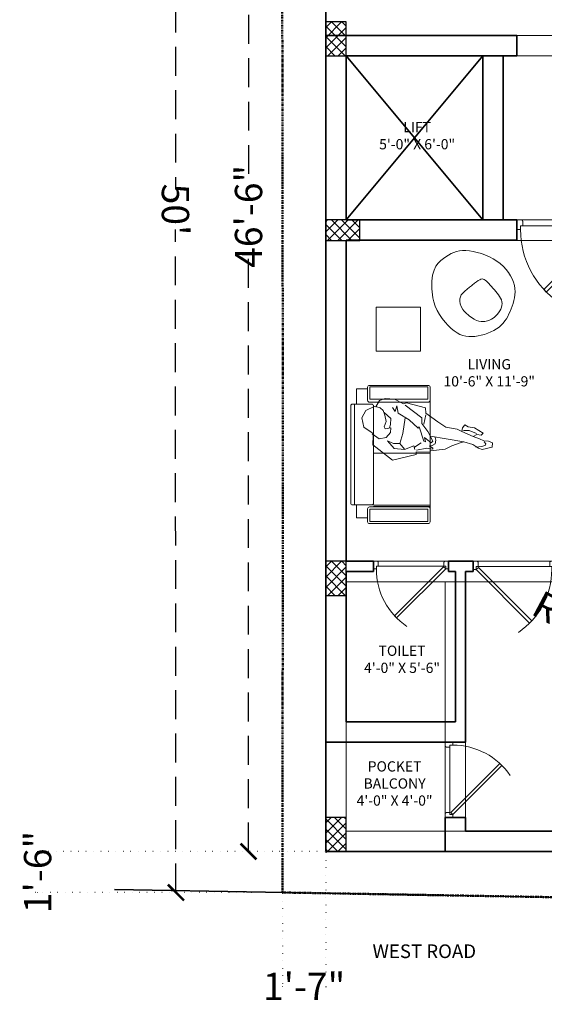
# Model space of a CAD drawing. Units: inches. Extents: x -16911 to -9621, y -48626 to -46270.
# Tile 17 of 20: x -11596 to -11365, y -47012 to -46579. Entities that reach past the tile are written whole.
import ezdxf

# ---------------------------------------------------------------- set-up
doc = ezdxf.new("R2010")
doc.units = ezdxf.units.IN
for name, pattern in [('DASHDOT', [1, 0.5, -0.25, 0, -0.25]), ('DASHED', [19.05, 12.7, -6.35]), ('DOT2', [3.175, 0, -3.175])]:
    doc.linetypes.add(name, pattern=pattern)
for name, color, linetype, lineweight in [('A-ANNO-DIMS', 2, 'Continuous', 13), ('A-ANNO-TEXT', 7, 'Continuous', 18), ('A-AREA-IDEN', 3, 'Continuous', 18), ('A-DOOR', 4, 'Continuous', 18), ('A-FURN', 8, 'Continuous', 13), ('A-WALL', 7, 'Continuous', 35), ('C-PROP', 6, 'DASHDOT', 50), ('column', 12, 'Continuous', 30), ('DOOR', 143, 'Continuous', 9), ('EXT BEAM', 132, 'Continuous', 13), ('furniture', 35, 'Continuous', 15), ('Man', 8, 'Continuous', 5), ('S-BEAM', 132, 'Continuous', 25), ('S-COLS', 1, 'Continuous', 30)]:
    doc.layers.add(name, color=color, linetype=linetype, lineweight=lineweight)
doc.styles.add('style9', font='swisscl.ttf', dxfattribs={"height": 12})
doc.dimstyles.new('Dim9', dxfattribs={"dimtxt": 10, "dimasz": 0.199219, "dimexe": 1, "dimexo": 0.5, "dimgap": 1, "dimtad": 0, "dimdec": 1, "dimzin": 0, "dimdsep": 46, "dimlunit": 4, "dimtxsty": 'style9', "dimblk": 'ARCHTICK', "dimcen": 0.09, "dimclrd": 256, "dimclrt": 256, "dimadec": 0, "dimazin": 0, "dimtfac": 1, "dimtdec": 1, "dimtix": 1, "dimtofl": 0, "dimtmove": 1, "dimatfit": 3, "dimfxl": 9, "dimtolj": 1, "dimtzin": 0, "dimlwd": -1, "dimarcsym": 0})

# ---------------------------------------------------------------- blocks, each defined once
blk = doc.blocks.new('Bipman02')
blk.add_lwpolyline([(0.5871, -0.067), (0.6175, -0.0496), (0.6523, -0.0539), (0.6697, -0.0376), (0.5958, 0.0069), (0.5437, 0.0156), (0.5164, 0.0297), (0.4959, 0.0069), (0.4915, -0.0235), (0.4524, -0.0061), (0.3568, 0.0113), (0.2917, 0.0548), (0.1917, 0.1287), (0.1874, 0.1722), (0.031, 0.2156), (0.0049, 0.2069), (-0.0689, 0.2461), (-0.1471, 0.2504), (-0.1949, 0.233), (-0.2253, 0.1808), (-0.2384, 0.1852), (-0.3079, 0.1504), (-0.3426, 0.0895), (-0.3253, 0.0113), (-0.2558, -0.0365), (-0.2471, -0.0583), (-0.2514, -0.1365), (-0.0863, -0.2626), (0.1092, -0.2148), (0.1092, -0.193), (0.2265, -0.1974), (0.2308, -0.1844), (0.3525, -0.1713), (0.409, -0.1452), (0.4872, -0.1148), (0.5089, -0.1104), (0.5828, -0.1322), (0.6088, -0.1496), (0.6295, -0.1636), (0.661, -0.1757), (0.7435, -0.1539), (0.7478, -0.1191), (0.7143, -0.1051), (0.674, -0.1017), (0.6392, -0.0844)], close=True)
for points in [[(-0.2558, -0.0452), (-0.1993, -0.0844), (-0.1385, -0.0757), (-0.1037, -0.0322), (-0.0994, 0.0069), (-0.1471, -0.0018), (-0.1558, 0.0156), (-0.1385, 0.0591), (-0.1515, 0.1113), (-0.1645, 0.1504), (-0.1906, 0.1722), (-0.2167, 0.1808)], [(-0.0863, 0.1765), (-0.0646, 0.1417), (-0.0516, 0.1895), (-0.0385, 0.1287), (0.0527, 0.0722), (0.1266, 0.0026), (0.1353, 0.0156), (0.1744, -0.1061), (0.1874, -0.1104), (0.1787, -0.0757), (0.2352, -0.1191), (0.2482, -0.1061), (0.2091, -0.0235), (0.157, 0.0417), (0.157, 0.0895), (0.018, 0.1939)], [(-0.1558, 0.133), (-0.0994, 0.0852), (-0.1037, 0.033), (-0.1124, 0.0069)], [(0.018, 0.0895), (0.0006, -0.0409), (-0.0255, -0.1235), (-0.0776, -0.1235), (-0.1298, -0.1017), (-0.0733, -0.167), (0.0136, -0.1757), (0.0918, -0.1452), (0.1005, -0.1757)], [(0.1917, 0.1156), (0.1744, 0.0374)], [(0.2699, -0.0757), (0.2743, -0.0974), (0.2699, -0.1278), (0.2439, -0.1409), (0.2222, -0.1452), (0.2482, -0.1626), (0.2482, -0.1713), (0.2004, -0.1626), (0.1135, -0.18)], [(0.2308, -0.0626), (0.3612, -0.0844), (0.5089, -0.1095)], [(0.4915, -0.0235), (0.5871, -0.067)], [(0.5045, -0.0148), (0.5523, -0.0148), (0.6132, -0.0409)], [(-0.0255, -0.1235), (0.0136, -0.1713)], [(0.0962, -0.1539), (0.1526, -0.1191)], [(0.6783, -0.1104), (0.6914, -0.1278), (0.687, -0.1409), (0.6566, -0.1496), (0.6088, -0.1539)]]:
    blk.add_lwpolyline(points)
blk = doc.blocks.new('erertety')
at = {"layer": 'furniture', "ltscale": 0.2}
for p, q in [((-17662.13, -45230.66), (-17662.13, -45176.69)), ((-17693.83, -45223.2), (-17693.83, -45184.43)), ((-17685.49, -45183.68), (-17693.08, -45183.68)), ((-17684.74, -45223.2), (-17684.74, -45184.43)), ((-17684.74, -45203.31), (-17662.13, -45203.31)), ((-17685.49, -45223.95), (-17693.08, -45223.95)), ((-17691.58, -45223.95), (-17691.58, -45229.1)), ((-17684.74, -45223.99), (-17662.13, -45223.99)), ((-17684.74, -45224.55), (-17662.13, -45224.55)), ((-17684.74, -45224.55), (-17662.13, -45224.55)), ((-17691.58, -45229.1), (-17687.09, -45229.1))]:
    blk.add_line(p, q, dxfattribs=at)
for points in [[(-17662.13, -45182.17), (-17662.13, -45176.97, 0.414214), (-17662.87, -45176.22), (-17686.34, -45176.22, 0.414214), (-17687.09, -45176.97), (-17687.09, -45182.17, 0.414214), (-17686.34, -45182.91), (-17662.87, -45182.91, 0.414214)], [(-17662.13, -45225.47), (-17662.13, -45230.66, -0.414214), (-17662.87, -45231.41), (-17686.34, -45231.41, -0.414214), (-17687.09, -45230.66), (-17687.09, -45225.47, -0.414214), (-17686.34, -45224.72), (-17662.87, -45224.72, -0.414214)]]:
    blk.add_lwpolyline(points, format="xyb", close=True, dxfattribs=at)
for points in [[(-17663.01, -45181.75), (-17663.01, -45176.82), (-17686.21, -45176.82), (-17686.21, -45181.75)], [(-17692.4, -45183.68), (-17692.4, -45223.95), (-17692.4, -45223.95), (-17692.4, -45183.68)], [(-17663.01, -45225.6), (-17663.01, -45230.53), (-17686.21, -45230.53), (-17686.21, -45225.6)]]:
    blk.add_lwpolyline(points, close=True, dxfattribs=at)
blk.add_lwpolyline([(-17687.09, -45177.54), (-17691.58, -45177.54), (-17691.58, -45183.68)], dxfattribs=at)
for centre, start, end in [((-17693.08, -45184.43), 90, 180), ((-17685.49, -45184.43), 0, 90), ((-17693.08, -45223.2), 180, 270), ((-17685.49, -45223.2), 270, 0)]:
    blk.add_arc(centre, 0.748, start, end, dxfattribs=at)
at = {"layer": 'furniture', "ltscale": 0.2, "xscale": 47.90818138957024, "yscale": 47.90818138957024, "zscale": 47.90818138957024}
blk.add_blockref('Bipman02', (-17673, -45193.44, 0), dxfattribs=at)
blk = doc.blocks.new('rthrty')
at = {"layer": 'furniture'}
blk.add_open_spline([(-17650.3, -45154.53), (-17651.97, -45142.9), (-17645.3, -45136.31), (-17637.11, -45132.37), (-17620.71, -45137.17), (-17612.47, -45149.45), (-17615.73, -45159.71), (-17619.67, -45168.02), (-17632.28, -45172.65), (-17641.84, -45170.43), (-17649.5, -45159.42), (-17650.3, -45154.53)], degree=3, dxfattribs=at)
at = {"layer": 'Man'}
blk.add_open_spline([(-17632.99, -45149.02), (-17629.89, -45146.6), (-17628, -45145.12), (-17623.29, -45151.15), (-17618.06, -45156.77), (-17623.15, -45164.08), (-17628.28, -45165.32), (-17631.61, -45164.6), (-17638.01, -45159.61), (-17638.81, -45154.69), (-17636.9, -45151.81), (-17632.99, -45149.02), (-17632.99, -45149.02)], degree=3, dxfattribs=at)
blk = doc.blocks.new('A$C1C9D3E54')
at = {"layer": 'DOOR'}
blk.add_line((18676.53, 5780.72), (18710.53, 5780.72), dxfattribs=at)
blk.add_lwpolyline([(18685.01, 5806.62), (18710.47, 5781.16), (18711.53, 5782.22), (18686.07, 5807.68), (18685.01, 5806.62)], dxfattribs=at)
blk.add_lwpolyline([(18674.03, 5778.22), (18676.03, 5778.22), (18674.03, 5778.22), (18674.03, 5782.22), (18675.53, 5782.22), (18675.53, 5780.72), (18676.53, 5780.72), (18676.53, 5778.72), (18676.41, 5778.72), (18676.41, 5778.6, -0.414214), (18676.16, 5778.35), (18676.03, 5778.35), (18676.03, 5778.22)], format="xyb", dxfattribs=at)
blk.add_lwpolyline([(18713.03, 5782.22), (18711.53, 5782.22), (18711.53, 5780.72), (18710.53, 5780.72), (18710.53, 5778.72), (18710.66, 5778.72), (18710.66, 5778.6, 0.414214), (18710.91, 5778.35), (18711.03, 5778.35), (18711.03, 5778.22), (18713.03, 5778.22), (18711.03, 5778.22), (18713.03, 5778.22), (18713.03, 5782.22)], format="xyb", close=True, dxfattribs=at)
blk.add_arc((18711.53, 5782.22), 36, 124.0336, 180, dxfattribs=at)
blk = doc.blocks.new('_ArchTick')
at = {"color": 0, "linetype": 'ByBlock', "const_width": 0.15}
blk.add_lwpolyline([(-0.5, -0.5), (0.5, 0.5)], dxfattribs=at)
blk = doc.blocks.new('*D13')
at = {"layer": 'A-ANNO-DIMS', "color": 0, "linetype": 'DOT2', "lineweight": -2, "transparency": 16777216}
for p, q in [((-11527.5, -46362.82), (-11528.69, -46362.82)), ((-11527.14, -46962.82), (-11528.32, -46962.82))]:
    blk.add_line(p, q, dxfattribs=at)
at = {"layer": 'A-ANNO-DIMS', "color": 0, "linetype": 'DASHED', "lineweight": 25, "transparency": 16777216}
for p, q in [((-11527.69, -46362.82), (-11527.51, -46653.98)), ((-11527.32, -46962.82), (-11527.5, -46671.67))]:
    blk.add_line(p, q, dxfattribs=at)
at = {"layer": 'Defpoints', "color": 0, "transparency": 16777216}
for p in [(-11527.69, -46362.82), (-11508.87, -46362.81), (-11508.51, -46962.81)]:
    blk.add_point(p, dxfattribs=at)
at = {"layer": 'A-ANNO-DIMS', "color": 0, "lineweight": 25, "transparency": 16777216, "xscale": 7, "yscale": 7, "zscale": 7}
for p, rotation in [((-11527.69, -46362.82), 90.0346840750536), ((-11527.32, -46962.82), 270.0346840750536)]:
    blk.add_blockref('_ArchTick', p, dxfattribs=dict(at, rotation=rotation))
at = {"layer": 'A-ANNO-DIMS', "color": 0, "transparency": 16777216, "insert": (-11527.51, -46662.82), "char_height": 12, "attachment_point": 5, "rotation": 270.0347, "style": 'style9'}
blk.add_mtext("\\A1;50'", dxfattribs=at)
blk = doc.blocks.new('*D15')
at = {"layer": 'A-ANNO-DIMS', "color": 0, "linetype": 'DOT2', "lineweight": -2, "transparency": 16777216}
for p, q in [((-11495.22, -46386.86), (-11496.4, -46386.86)), ((-11495.22, -46944.81), (-11496.4, -46944.81))]:
    blk.add_line(p, q, dxfattribs=at)
at = {"layer": 'A-ANNO-DIMS', "color": 0, "linetype": 'DASHED', "lineweight": 25, "transparency": 16777216}
for p, q in [((-11495.4, -46386.86), (-11495.4, -46648.2)), ((-11495.4, -46944.81), (-11495.4, -46683.47))]:
    blk.add_line(p, q, dxfattribs=at)
at = {"layer": 'Defpoints', "color": 0, "transparency": 16777216}
for p in [(-11461.47, -46386.86), (-11495.4, -46944.81), (-11461.47, -46944.81)]:
    blk.add_point(p, dxfattribs=at)
at = {"layer": 'A-ANNO-DIMS', "color": 0, "lineweight": 25, "transparency": 16777216, "xscale": 7, "yscale": 7, "zscale": 7}
for p, rotation in [((-11495.4, -46386.86), 90), ((-11495.4, -46944.81), 270)]:
    blk.add_blockref('_ArchTick', p, dxfattribs=dict(at, rotation=rotation))
at = {"layer": 'A-ANNO-DIMS', "color": 0, "transparency": 16777216, "insert": (-11495.4, -46665.83), "char_height": 12, "attachment_point": 5, "rotation": 90, "style": 'style9'}
blk.add_mtext('\\A1;46\'-6"', dxfattribs=at)
blk = doc.blocks.new('COLUMNS')
at = {"layer": 'column'}
h = blk.add_hatch(dxfattribs=at)
h.set_pattern_fill('ANSI37', color=256, angle=-900)
h.set_pattern_definition([(225, (-45817.4075, 11499.4594), (2.24506403, -2.24506403), []), (315, (-45817.4075, 11499.4594), (2.24506403, 2.24506403), [])])
h.paths.add_polyline_path([(-12052.47, -46580.36), (-12061.47, -46580.36), (-12061.47, -46595.36), (-12052.47, -46595.36)])
h = blk.add_hatch(dxfattribs=at)
h.set_pattern_fill('ANSI37', color=256, angle=-810)
h.set_pattern_definition([(315, (-70141.2892, -80432.2886), (2.24506403, 2.24506403), []), (45, (-70141.2892, -80432.2886), (-2.24506403, 2.24506403), [])])
h.paths.add_polyline_path([(-12061.47, -46667.36), (-12061.47, -46676.36), (-12046.47, -46676.36), (-12046.47, -46667.36)])
h = blk.add_hatch(dxfattribs=at)
h.set_pattern_fill('ANSI37', color=256, angle=-540)
h.set_pattern_definition([(225, (-45817.4075, 11262.5055), (2.24506403, -2.24506403), []), (315, (-45817.4075, 11262.5055), (2.24506403, 2.24506403), [])])
h.paths.add_polyline_path([(-12052.47, -46817.31), (-12061.47, -46817.31), (-12061.47, -46832.31), (-12052.47, -46832.31)])
h = blk.add_hatch(dxfattribs=at)
h.set_pattern_fill('ANSI37', color=256, angle=-720)
h.set_pattern_definition([(45, (21703.4588, -105024.6242), (-2.24506403, 2.24506403), []), (135, (21703.4588, -105024.6242), (-2.24506403, -2.24506403), [])])
h.paths.add_polyline_path([(-12061.47, -46944.81), (-12052.47, -46944.81), (-12052.47, -46929.81), (-12061.47, -46929.81)])
at = {"layer": 'column', "ltscale": 0.05}
for points in [[(-12061.47, -46595.36), (-12052.47, -46595.36), (-12052.47, -46580.36), (-12061.47, -46580.36)], [(-12046.47, -46676.36), (-12046.47, -46667.36), (-12061.47, -46667.36), (-12061.47, -46676.36)], [(-12061.47, -46832.31), (-12052.47, -46832.31), (-12052.47, -46817.31), (-12061.47, -46817.31)], [(-12052.47, -46929.81), (-12061.47, -46929.81), (-12061.47, -46944.81), (-12052.47, -46944.81)]]:
    blk.add_lwpolyline(points, close=True, dxfattribs=at)
blk = doc.blocks.new('3RD ROOF BEAMS')
at = {"layer": 'EXT BEAM'}
for p, q in [((-11461.47, -46586.36), (-11324.72, -46586.36)), ((-11461.47, -46944.81), (-11461.47, -46586.36)), ((-11320.47, -46586.36), (-11138.92, -46586.36)), ((-11138.92, -46944.81), (-11138.92, -46586.36)), ((-11452.47, -46595.36), (-11324.72, -46595.36)), ((-11392.47, -46595.36), (-11392.47, -46667.36)), ((-11383.47, -46595.36), (-11383.47, -46667.36)), ((-11320.47, -46595.36), (-11147.92, -46595.36)), ((-11302.92, -46595.36), (-11302.92, -46667.36)), ((-11293.92, -46595.36), (-11293.92, -46667.36)), ((-11147.92, -46667.36), (-11147.92, -46595.36)), ((-11446.47, -46667.36), (-11335.47, -46667.36)), ((-11320.47, -46667.36), (-11138.92, -46667.36)), ((-11452.47, -46817.31), (-11452.47, -46676.36)), ((-11446.47, -46676.36), (-11335.47, -46676.36)), ((-11324.97, -46676.36), (-11324.97, -46817.31)), ((-11320.47, -46676.36), (-11138.92, -46676.36)), ((-11315.97, -46676.36), (-11315.97, -46817.31)), ((-11195.92, -46676.36), (-11195.92, -46764.81)), ((-11186.92, -46676.36), (-11186.92, -46764.81)), ((-11147.92, -46817.31), (-11147.92, -46676.36)), ((-11147.92, -46764.81), (-11315.97, -46764.81)), ((-11147.92, -46773.81), (-11315.97, -46773.81)), ((-11452.47, -46817.31), (-11147.92, -46817.31)), ((-11452.47, -46826.31), (-11279.72, -46826.31)), ((-11452.47, -46944.81), (-11452.47, -46826.31)), ((-11408.97, -46826.31), (-11408.97, -46935.81)), ((-11399.97, -46826.31), (-11399.97, -46935.81)), ((-11279.72, -46826.31), (-11279.72, -46935.81)), ((-11270.72, -46826.31), (-11147.92, -46826.31)), ((-11270.72, -46826.31), (-11270.72, -46935.81)), ((-11147.92, -46935.81), (-11147.92, -46826.31)), ((-11452.47, -46935.81), (-11279.72, -46935.81)), ((-11270.72, -46935.81), (-11147.92, -46935.81)), ((-11461.47, -46944.81), (-11138.92, -46944.81))]:
    blk.add_line(p, q, dxfattribs=at)
blk = doc.blocks.new('*D128')
at = {"layer": 'A-ANNO-DIMS', "color": 0, "linetype": 'DOT2', "lineweight": -2, "transparency": 16777216}
for p, q in [((-11461.97, -46944.81), (-11589.1, -46944.81)), ((-11480.97, -46962.81), (-11589.1, -46962.81))]:
    blk.add_line(p, q, dxfattribs=at)
at = {"layer": 'A-ANNO-DIMS', "linetype": 'DASHED', "transparency": 16777216}
for p, q in [((-11588.1, -46944.81), (-11588.1, -46944.61)), ((-11588.1, -46962.81), (-11588.1, -46963.01))]:
    blk.add_line(p, q, dxfattribs=at)
at = {"layer": 'Defpoints', "color": 0, "transparency": 16777216}
for p in [(-11588.1, -46944.81), (-11461.47, -46944.81), (-11480.47, -46962.81)]:
    blk.add_point(p, dxfattribs=at)
at = {"layer": 'A-ANNO-DIMS', "transparency": 16777216, "xscale": 0.19921875, "yscale": 0.19921875, "zscale": 0.19921875}
for p, rotation in [((-11588.1, -46944.81), 270), ((-11588.1, -46962.81), 90)]:
    blk.add_blockref('_ArchTick', p, dxfattribs=dict(at, rotation=rotation))
at = {"layer": 'A-ANNO-DIMS', "transparency": 16777216, "insert": (-11588.1, -46953.81), "char_height": 12, "attachment_point": 5, "rotation": 90, "style": 'style9'}
blk.add_mtext('\\A1;1\'-6"', dxfattribs=at)
blk = doc.blocks.new('*D130')
at = {"layer": 'A-ANNO-DIMS', "color": 0, "linetype": 'DOT2', "lineweight": -2, "transparency": 16777216}
for p, q in [((-11461.47, -46945.31), (-11461.47, -47005.04)), ((-11480.47, -46963.31), (-11480.47, -47005.04))]:
    blk.add_line(p, q, dxfattribs=at)
at = {"layer": 'A-ANNO-DIMS', "linetype": 'DASHED', "transparency": 16777216}
for p, q in [((-11480.47, -47004.04), (-11480.67, -47004.04)), ((-11461.47, -47004.04), (-11461.28, -47004.04))]:
    blk.add_line(p, q, dxfattribs=at)
at = {"layer": 'Defpoints', "color": 0, "transparency": 16777216}
for p in [(-11461.47, -46944.81), (-11480.47, -46962.81), (-11461.47, -47004.04)]:
    blk.add_point(p, dxfattribs=at)
at = {"layer": 'A-ANNO-DIMS', "transparency": 16777216, "xscale": 0.19921875, "yscale": 0.19921875, "zscale": 0.19921875}
blk.add_blockref('_ArchTick', (-11480.47, -47004.04), dxfattribs=at)
at = {"layer": 'A-ANNO-DIMS', "transparency": 16777216, "xscale": 0.19921875, "yscale": 0.19921875, "zscale": 0.19921875, "rotation": 180}
blk.add_blockref('_ArchTick', (-11461.47, -47004.04), dxfattribs=at)
at = {"layer": 'A-ANNO-DIMS', "transparency": 16777216, "insert": (-11470.97, -47004.04), "char_height": 12, "attachment_point": 5, "style": 'style9'}
blk.add_mtext('\\A1;1\'-7"', dxfattribs=at)
blk = doc.blocks.new('*D137')
at = {"layer": 'A-ANNO-DIMS', "color": 0, "lineweight": -2, "transparency": 16777216}
for p, q in [((-11395.43, -46821), (-11395.25, -46821)), ((-11395.34, -46821.09), (-11395.34, -46820.91))]:
    blk.add_line(p, q, dxfattribs=at)
at = {"layer": 'A-ANNO-DIMS', "linetype": 'DASHED', "transparency": 16777216}
blk.add_line((-11364.07, -46837.61), (-11365.99, -46836.59), dxfattribs=at)
at = {"layer": 'Defpoints', "color": 0, "transparency": 16777216}
for p in [(-11395.34, -46821), (-11365.99, -46836.59)]:
    blk.add_point(p, dxfattribs=at)
at = {"layer": 'A-ANNO-DIMS', "transparency": 16777216, "xscale": 0.19921875, "yscale": 0.19921875, "zscale": 0.19921875, "rotation": 152.0175078160649}
blk.add_blockref('_ArchTick', (-11365.99, -46836.59), dxfattribs=at)
at = {"layer": 'A-ANNO-DIMS', "transparency": 16777216, "insert": (-11348.39, -46845.95), "char_height": 12, "attachment_point": 5, "rotation": 332.0175, "style": 'style9'}
blk.add_mtext('\\A1;R2\'-9"', dxfattribs=at)

msp = doc.modelspace()

# ---------------------------------------------------------------- linework, layer by layer
at = {"layer": 'A-FURN'}
msp.add_lwpolyline([(-11419.878, -46705.751), (-11439.238, -46705.751), (-11439.238, -46725.111), (-11419.878, -46725.111)], close=True, dxfattribs=at)
at = {"layer": 'A-WALL'}
for p, q in [((-11461.474, -46586.355), (-11461.474, -46386.855)), ((-11461.474, -46896.809), (-11461.474, -46586.355)), ((-11377.474, -46586.355), (-11461.474, -46586.355)), ((-11377.474, -46595.355), (-11377.474, -46586.355)), ((-11452.474, -46667.355), (-11452.474, -46595.355)), ((-11377.474, -46595.355), (-11452.474, -46595.355)), ((-11452.474, -46595.355), (-11392.474, -46667.355)), ((-11452.474, -46667.355), (-11392.474, -46595.355)), ((-11392.474, -46667.355), (-11392.474, -46595.355)), ((-11383.474, -46667.355), (-11383.474, -46595.355)), ((-11377.474, -46667.355), (-11452.474, -46667.355)), ((-11377.474, -46676.355), (-11377.474, -46667.355)), ((-11452.474, -46817.309), (-11452.474, -46676.355)), ((-11377.474, -46676.355), (-11452.474, -46676.355)), ((-11452.474, -46817.309), (-11440.474, -46817.309)), ((-11440.474, -46817.309), (-11440.474, -46821.809)), ((-11407.474, -46817.309), (-11396.724, -46817.309)), ((-11407.474, -46817.309), (-11407.474, -46821.809)), ((-11396.724, -46821.809), (-11396.724, -46817.309)), ((-11452.474, -46887.809), (-11452.474, -46821.809)), ((-11452.474, -46821.809), (-11440.474, -46821.809)), ((-11407.474, -46821.809), (-11404.474, -46821.809)), ((-11404.474, -46887.809), (-11404.474, -46821.809)), ((-11399.974, -46896.809), (-11399.974, -46821.809)), ((-11399.974, -46821.809), (-11396.724, -46821.809)), ((-11452.474, -46887.809), (-11404.474, -46887.809)), ((-11461.474, -46944.809), (-11461.474, -46896.809)), ((-11461.474, -46896.809), (-11399.974, -46896.809)), ((-11408.974, -46944.809), (-11408.974, -46929.809)), ((-11408.974, -46929.809), (-11399.974, -46929.809)), ((-11399.974, -46935.809), (-11399.974, -46929.809)), ((-11399.974, -46935.809), (-11279.724, -46935.809)), ((-11461.474, -46944.809), (-11408.974, -46944.809)), ((-11408.974, -46944.809), (-11138.925, -46944.809)), ((-11047.547, -46970.292), (-11554.349, -46961.533))]:
    msp.add_line(p, q, dxfattribs=at)
at = {"layer": 'C-PROP'}
msp.add_lwpolyline([(-11480.474, -46962.809), (-11120.293, -46969.035), (-11119.732, -46940.446), (-11120.395, -46855.606), (-11121.561, -46609.511), (-11121.175, -46367.855), (-11480.838, -46362.811), (-11480.3, -46762.955)], close=True, dxfattribs=at)

# ---------------------------------------------------------------- block references
at = {"layer": 'A-DOOR'}
for p, xscale, yscale, zscale, rotation in [((-31487.969, -40444.653), -1.076923076922859, 1.076923076922859, 1.076923076922859, 180), ((-27241.577, -41928.043), -0.8461538461538624, 0.8461538461538624, 0.8461538461538624, 180), ((5876.842, -41483.564), 0.9230769230769229, 0.9230769230769229, 0.9230769230769229, 180), ((-16298.241, -31095.706), 0.8461538461538624, 0.8461538461538624, 0.8461538461538624, 270)]:
    msp.add_blockref('A$C1C9D3E54', p, dxfattribs=dict(at, xscale=xscale, yscale=yscale, zscale=zscale, rotation=rotation))
at = {"layer": 'A-FURN'}
msp.add_blockref('rthrty', (6235.852, -1547.053), dxfattribs=at)
at = {"layer": 'A-FURN', "xscale": 1.1, "yscale": 1.1, "zscale": 1.1}
msp.add_blockref('erertety', (8012.76, 2953.75, 0), dxfattribs=at)
at = {"layer": 'S-BEAM'}
msp.add_blockref('3RD ROOF BEAMS', (0, 0), dxfattribs=at)
at = {"layer": 'S-COLS'}
msp.add_blockref('COLUMNS', (600, 0), dxfattribs=at)

# ---------------------------------------------------------------- texts
at = {"layer": 'A-ANNO-TEXT', "ltscale": 10, "insert": (-11440.885, -46985.611), "char_height": 6, "width": 70.69764, "attachment_point": 1, "style": 'style9'}
msp.add_mtext('\\A1;{\\fCentury Gothic|b0|i0|c0|p34;WEST ROAD}', dxfattribs=at)
at = {"layer": 'A-AREA-IDEN', "ltscale": 10, "char_height": 4.5, "width": 42.823, "attachment_point": 1, "style": 'style9'}
for s, insert in [('\\A1;\\pxqc;{\\fCentury Gothic|b0|i0|c0|p34;LIFT\\P5\'-0" X 6\'-0"}', (-11442.698, -46624.39)), ('\\A1;\\pxqc;{\\fCentury Gothic|b0|i0|c0|p34;LIVING\\P10\'-6" X 11\'-9"}', (-11411.012, -46728.541)), ('\\A1;\\pxqc;{\\fCentury Gothic|b0|i0|c0|p34;TOILET\\P4\'-0" X 5\'-6"}', (-11449.33, -46854.373)), ('\\A1;\\pxqc;{\\fCentury Gothic|b0|i0|c0|p34;POCKET BALCONY\\P4\'-0" X 4\'-0"}', (-11452.615, -46905.176))]:
    msp.add_mtext(s, dxfattribs=dict(at, insert=insert))

# ---------------------------------------------------------------- dimensions: what is measured, and where the dimension line sits
at = {"layer": 'A-ANNO-DIMS'}
dim = msp.add_aligned_dim(p1=(-11508.507, -46962.809), p2=(-11508.87, -46362.811), distance=18.817, dimstyle='Dim9', override={"dimtxt": 12, "dimasz": 7, "dimdec": 2, "dimclrd": 0, "dimclre": 0, "dimclrt": 0, "dimtdec": 2, "dimfxl": 0.1875, "dimfxlon": 1, "dimlwd": 25, "dimarcsym": 2}, dxfattribs=at)
dim.commit()
dim.dimension.update_dxf_attribs({"geometry": '*D13', "text_midpoint": (-11527.505, -46662.821)})
for base, p1, override, picture, middle in [((-11495.403, -46944.809), (-11461.474, -46386.855), {"dimtxt": 12, "dimasz": 7, "dimdec": 2, "dimclrd": 0, "dimclre": 0, "dimclrt": 0, "dimtdec": 2, "dimfxl": 0.1875, "dimfxlon": 1, "dimlwd": 25, "dimarcsym": 2}, '*D15', (-11495.403, -46665.832)), ((-11588.099, -46944.809), (-11480.474, -46962.809), {"dimdec": 1, "dimlfac": 1, "dimrnd": 0, "dimzin": 1, "dimdsep": 46, "dimlunit": 4, "dimfrac": 2}, '*D128', (-11588.099, -46953.809))]:
    dim = msp.add_linear_dim(base=base, p1=p1, p2=(-11461.474, -46944.809), angle=90, dimstyle='Dim9', override=override, dxfattribs=at)
    dim.commit()
    dim.dimension.update_dxf_attribs({"geometry": picture, "text_midpoint": middle})
dim = msp.add_radius_dim(center=(-11395.34, -46820.998), mpoint=(-11365.994, -46836.59), dimstyle='Dim9', override={"dimdec": 1, "dimlfac": 1, "dimrnd": 0, "dimzin": 1, "dimdsep": 46, "dimlunit": 4, "dimfrac": 2}, dxfattribs=at)
dim.commit()
dim.dimension.update_dxf_attribs({"geometry": '*D137', "text_midpoint": (-11348.386, -46845.945), "dimtype": 164})
dim = msp.add_linear_dim(base=(-11461.474, -47004.042), p1=(-11480.474, -46962.809), p2=(-11461.474, -46944.809), dimstyle='Dim9', override={"dimdec": 1, "dimlfac": 1, "dimrnd": 0, "dimzin": 1, "dimdsep": 46, "dimlunit": 4, "dimfrac": 2}, dxfattribs=at)
dim.commit()
dim.dimension.update_dxf_attribs({"geometry": '*D130', "text_midpoint": (-11470.974, -47004.042)})

doc.saveas('drawing.dxf')
